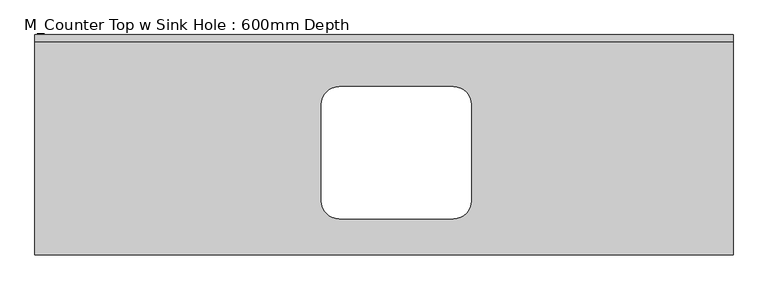
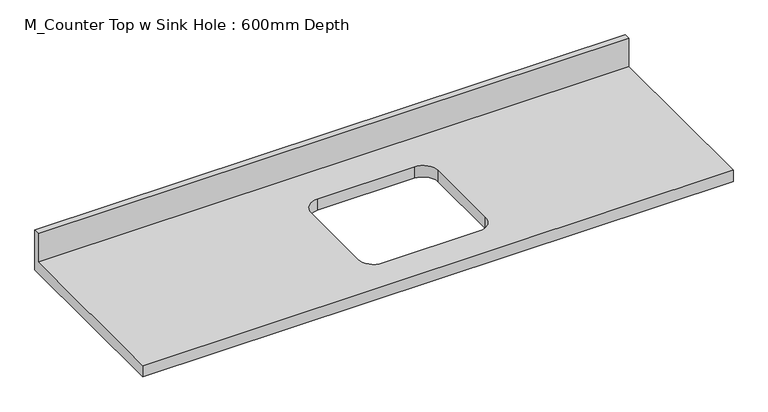
"""IFC4 building model written with IfcOpenShell, lengths in millimetres: furniture geometry, M_Counter Top w Sink Hole : 600mm Depth."""

from ifc_helpers import new_model, si_unit, frame, origin, place, context, project, spatial, polyline, circle_curve, source, transform, mapped, element, save
from ifc_brep_helpers import plane_surface, revolved_surface, advanced_brep


def m_counter_top_w_sink_hole_600mm_depth_0a237b63(model_context):
    return source(origin(), model_context, "Body", "AdvancedBrep", [
        advanced_brep(
        [(-1200.4622951, -625.0, 900.0), (779.5377049, -625.0, 900.0), (779.5377049, -19.05, 900.0), (-1200.4622951, -19.05, 900.0), (-337.3622951, -147.3, 900.0), (-13.5622951, -147.3, 900.0), (37.2377049, -198.1, 900.0), (37.2377049, -471.9, 900.0), (-13.5622951, -522.7, 900.0), (-337.3622951, -522.7, 900.0), (-388.1622951, -471.9, 900.0), (-388.1622951, -198.1, 900.0), (779.5377049, 0.0, 860.0), (779.5377049, -625.0, 860.0), (-1200.4622951, -625.0, 860.0), (-1200.4622951, 0.0, 860.0), (-13.5622951, -147.3, 860.0), (-337.3622951, -147.3, 860.0), (-388.1622951, -198.1, 860.0), (-388.1622951, -471.9, 860.0), (-337.3622951, -522.7, 860.0), (-13.5622951, -522.7, 860.0), (37.2377049, -471.9, 860.0), (37.2377049, -198.1, 860.0), (-1200.4622951, 0.0, 1001.6), (779.5377049, 0.0, 1001.6), (-1200.4622951, -19.05, 1001.6), (779.5377049, -19.05, 1001.6)],
        [
            (0, 1),
            (1, 2),
            (2, 3),
            (3, 0),
            (4, 5),
            (5, 6, circle_curve(frame((-13.5622951, -198.1, 900.0), z_axis=(0.0, 0.0, -1.0), x_axis=(1.0, 0.0, 0.0)), 50.8)),
            (6, 7),
            (7, 8, circle_curve(frame((-13.5622951, -471.9, 900.0), z_axis=(0.0, 0.0, -1.0), x_axis=(1.0, 0.0, 0.0)), 50.8)),
            (8, 9),
            (9, 10, circle_curve(frame((-337.3622951, -471.9, 900.0), z_axis=(0.0, 0.0, -1.0), x_axis=(1.0, 0.0, 0.0)), 50.8)),
            (10, 11),
            (11, 4, circle_curve(frame((-337.3622951, -198.1, 900.0), z_axis=(0.0, 0.0, -1.0), x_axis=(1.0, 0.0, 0.0)), 50.8)),
            (12, 13),
            (13, 14),
            (14, 15),
            (15, 12),
            (16, 17),
            (17, 18, circle_curve(frame((-337.3622951, -198.1, 860.0), z_axis=(0.0, 0.0, 1.0), x_axis=(1.0, 0.0, 0.0)), 50.8)),
            (18, 19),
            (19, 20, circle_curve(frame((-337.3622951, -471.9, 860.0), z_axis=(0.0, 0.0, 1.0), x_axis=(1.0, 0.0, 0.0)), 50.8)),
            (20, 21),
            (21, 22, circle_curve(frame((-13.5622951, -471.9, 860.0), z_axis=(0.0, 0.0, 1.0), x_axis=(1.0, 0.0, 0.0)), 50.8)),
            (22, 23),
            (23, 16, circle_curve(frame((-13.5622951, -198.1, 860.0), z_axis=(0.0, 0.0, 1.0), x_axis=(1.0, 0.0, 0.0)), 50.8)),
            (15, 24),
            (24, 25),
            (25, 12),
            (14, 0),
            (3, 26),
            (26, 24),
            (13, 1),
            (25, 27),
            (27, 2),
            (26, 27),
            (4, 17),
            (16, 5),
            (11, 18),
            (10, 19),
            (9, 20),
            (8, 21),
            (7, 22),
            (6, 23),
        ],
        [
            plane_surface(frame((-1200.4622951, 0.0, 900.0), z_axis=(0.0, 0.0, 1.0), x_axis=(-1.0, 0.0, 0.0))),
            plane_surface(frame((-1200.4622951, 0.0, 860.0), z_axis=(0.0, 0.0, -1.0), x_axis=(1.0, 0.0, 0.0))),
            plane_surface(frame((779.5377049, 0.0, 900.0), z_axis=(0.0, 1.0, 0.0), x_axis=(0.0, 0.0, -1.0))),
            plane_surface(frame((-1200.4622951, 0.0, 900.0), z_axis=(-1.0, 0.0, 0.0), x_axis=(0.0, 0.0, -1.0))),
            plane_surface(frame((-1200.4622951, -625.0, 900.0), z_axis=(0.0, -1.0, 0.0), x_axis=(0.0, 0.0, -1.0))),
            plane_surface(frame((779.5377049, -625.0, 900.0), z_axis=(1.0, 0.0, 0.0), x_axis=(0.0, 0.0, -1.0))),
            plane_surface(frame((-1200.4622951, 0.0, 1001.6), z_axis=(0.0, 0.0, 1.0), x_axis=(0.0, -1.0, 0.0))),
            plane_surface(frame((-1200.4622951, -19.05, 1001.6), z_axis=(0.0, -1.0, 0.0), x_axis=(0.0, 0.0, -1.0))),
            plane_surface(frame((-13.5622951, -147.3, 900.0), z_axis=(0.0, -1.0, 0.0), x_axis=(0.0, 0.0, -1.0))),
            revolved_surface(polyline([(-286.5622951, -198.1, 900.0), (-286.5622951, -198.1, 860.0)]), (-337.3622951, -198.1, 860.0), (0.0, 0.0, 1.0)),
            plane_surface(frame((-388.1622951, -198.1, 900.0), z_axis=(1.0, 0.0, 0.0), x_axis=(0.0, 0.0, -1.0))),
            revolved_surface(polyline([(-286.5622951, -471.9, 900.0), (-286.5622951, -471.9, 860.0)]), (-337.3622951, -471.9, 860.0), (0.0, 0.0, 1.0)),
            plane_surface(frame((-337.3622951, -522.7, 900.0), z_axis=(0.0, 1.0, 0.0), x_axis=(0.0, 0.0, -1.0))),
            revolved_surface(polyline([(37.2377049, -471.9, 900.0), (37.2377049, -471.9, 860.0)]), (-13.5622951, -471.9, 860.0), (0.0, 0.0, 1.0)),
            plane_surface(frame((37.2377049, -471.9, 900.0), z_axis=(-1.0, 0.0, 0.0), x_axis=(0.0, 0.0, -1.0))),
            revolved_surface(polyline([(37.2377049, -198.1, 900.0), (37.2377049, -198.1, 860.0)]), (-13.5622951, -198.1, 860.0), (0.0, 0.0, 1.0)),
        ],
        [
            (0, [[1, 2, 3, 4], [5, 6, 7, 8, 9, 10, 11, 12]]),
            (1, [[13, 14, 15, 16], [17, 18, 19, 20, 21, 22, 23, 24]]),
            (2, [[-16, 25, 26, 27]]),
            (3, [[-15, 28, -4, 29, 30, -25]]),
            (4, [[-1, -28, -14, 31]]),
            (5, [[-13, -27, 32, 33, -2, -31]]),
            (6, [[-30, 34, -32, -26]]),
            (7, [[-34, -29, -3, -33]]),
            (8, [[35, -17, 36, -5]]),
            (9, [[-35, -12, 37, -18]]),
            (10, [[-37, -11, 38, -19]]),
            (11, [[-38, -10, 39, -20]]),
            (12, [[-39, -9, 40, -21]]),
            (13, [[-40, -8, 41, -22]]),
            (14, [[-41, -7, 42, -23]]),
            (15, [[-36, -24, -42, -6]]),
        ],
    ),
    ])


if __name__ == "__main__":
    model = new_model("IFC4")
    model_context = context("Model", 3, world=origin())
    ifc_project = project(units=[si_unit("LENGTHUNIT", "METRE", prefix="MILLI")], contexts=[model_context])
    site = spatial("IfcSite", under=ifc_project)
    building = spatial("IfcBuilding", under=site)
    placement = place(None, origin())
    m_counter_top_w_sink_hole_600mm_depth_shape = m_counter_top_w_sink_hole_600mm_depth_0a237b63(model_context)
    element("IfcFurniture", 1, ObjectType="M_Counter Top w Sink Hole : 600mm Depth", at=placement, inside=building, context=model_context, shape_type="MappedRepresentation", body=[
        mapped(m_counter_top_w_sink_hole_600mm_depth_shape, transform((0.0, 0.0, 0.0), x_axis=(1.0, 0.0, 0.0), y_axis=(0.0, 1.0, 0.0), z_axis=(0.0, 0.0, 1.0))),
    ])
    save(model, "model.ifc")

# Revit data of these elements
# Type "M_Counter Top w Sink Hole : 600mm Depth"
#   Counter Thickness = 40 mm
#   Depth = 625 mm
#   Height = 900 mm
#   Length [instance default] = 2500 mm
#   Sink Location [instance default] = 1200 mm
#   Sink Location To Wall [instance default] = 100 mm
#   Sink Opening Depth [instance default] = 378 mm
#   Sink Opening Width [instance default] = 587 mm
#   Counter Top Material = none
#   Default Elevation = 0
# Element 1 (IfcFurniture, "M_Counter Top w Sink Hole : 600mm Depth")
#   Length = 1980 mm
#   Sink Location = 1025 mm
#   Sink Location To Wall = 160 mm
#   Sink Opening Depth = 350 mm
#   Sink Opening Width = 400 mm
#   Materials on its faces: "Counter Top"
# Materials
#   "Counter Top": class "Wood", colour RGB 226 177 128, transparency 0
